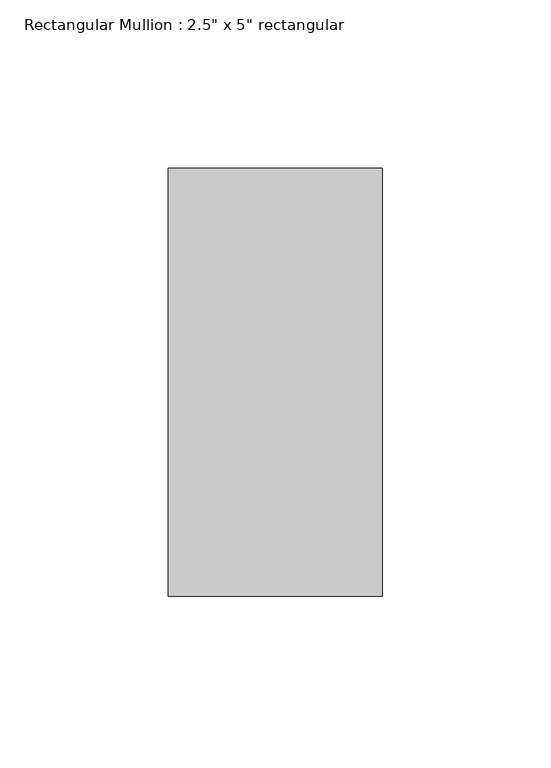
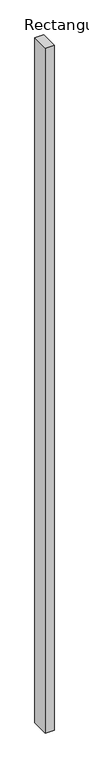
"""IFC4 building model written with IfcOpenShell, lengths in millimetres: member geometry."""

from ifc_helpers import new_model, si_unit, frame, origin, place, context, project, spatial, polyline, outline, extrude, source, transform, mapped, element, save


def member_1706ff29(model_context):
    return source(origin(), model_context, "Body", "SweptSolid", [
        extrude(outline(polyline([(31.75, 63.5), (31.75, -63.5), (-31.75, -63.5), (-31.75, 63.5), (31.75, 63.5)])), frame((0.0, 0.0, -5181.6), z_axis=(0.0, 0.0, 1.0), x_axis=(1.0, 0.0, 0.0)), (0.0, 0.0, 1.0), 5181.6),
    ])


if __name__ == "__main__":
    model = new_model("IFC4")
    model_context = context("Model", 3, world=origin())
    ifc_project = project(units=[si_unit("LENGTHUNIT", "METRE", prefix="MILLI")], contexts=[model_context])
    site = spatial("IfcSite", under=ifc_project)
    building = spatial("IfcBuilding", under=site)
    placement = place(None, origin())
    member_shape = member_1706ff29(model_context)
    element("IfcMember", 1, ObjectType="Rectangular Mullion : 2.5\" x 5\" rectangular", at=placement, inside=building, context=model_context, shape_type="MappedRepresentation", body=[
        mapped(member_shape, transform((0.0, 0.0, 0.0), x_axis=(1.0, 0.0, 0.0), y_axis=(0.0, 1.0, 0.0), z_axis=(0.0, 0.0, 1.0))),
    ])
    save(model, "model.ifc")

# Revit data of these elements
# Type "Rectangular Mullion : 2.5\" x 5\" rectangular"
#   built-in parameter 1007304 = 0.416667 (stored number, unit not read)
#   built-in parameter 1007301 = 0.104167 (stored number, unit not read)
#   built-in parameter 1007300 = 0.104167 (stored number, unit not read)
# Element 1 (IfcMember, "Rectangular Mullion : 2.5\" x 5\" rectangular")
#   Materials on its faces: "Iron, Ductile"
# Materials
#   "Iron, Ductile": class "Metal", colour RGB 0 0 0, transparency 0, Description = "Ductile cast iron", Cost = 0
